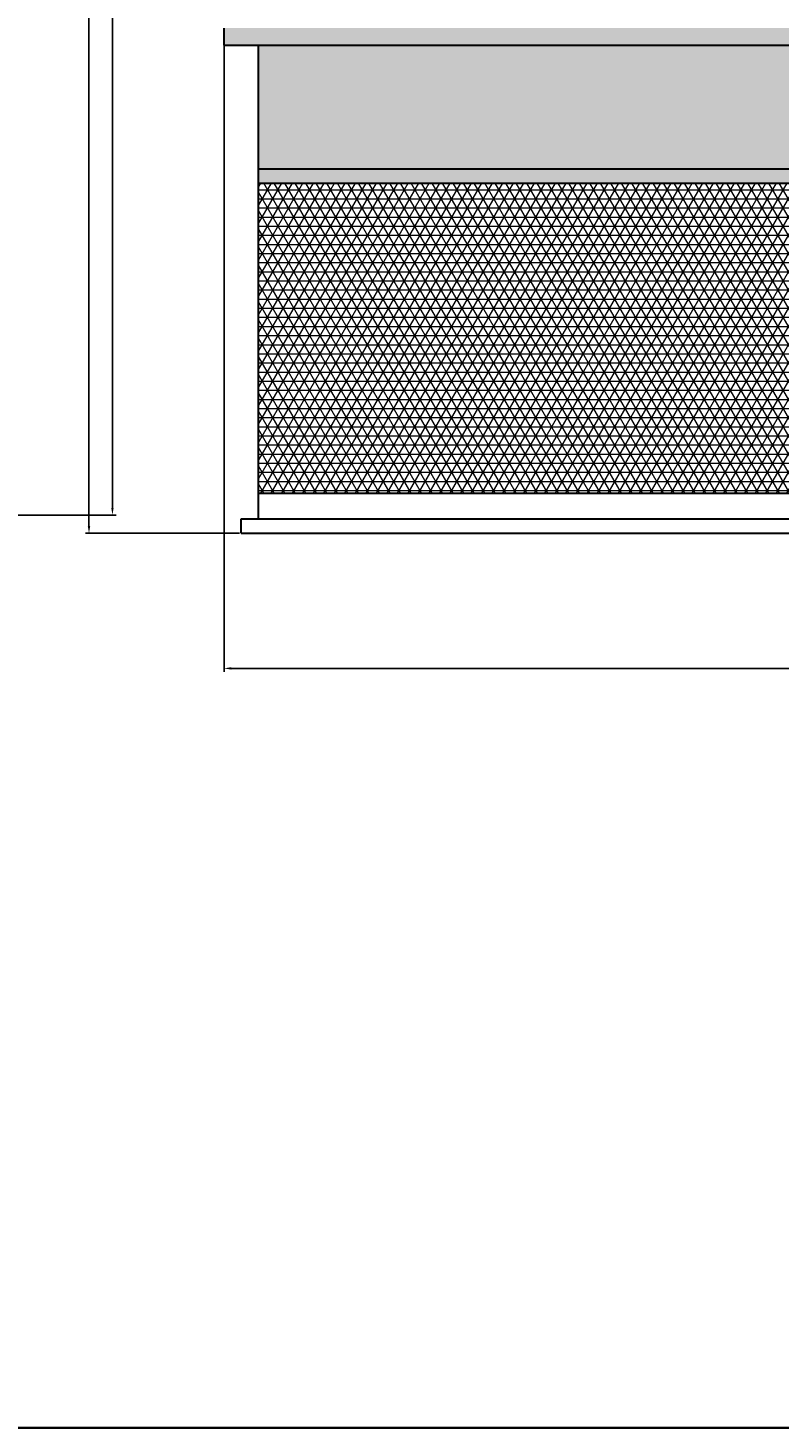
# Model space of a CAD drawing. Units: inches. Extents: x 2391 to 16591, y 7259 to 10239.
# Tile 11 of 27: x 3487 to 3749, y 7259 to 7746. Entities that reach past the tile are written whole.
import ezdxf

# ---------------------------------------------------------------- set-up
doc = ezdxf.new("R2010")
doc.units = ezdxf.units.IN
for name, color, linetype, lineweight in [('A-ANNO-DIMS', 4, 'Continuous', 18), ('A-ANNO-TTLB', 7, 'Continuous', 35), ('A-ELEV', 7, 'Continuous', 30), ('A-ELEV-PATT', 8, 'Continuous', 13), ('A-ELEV-SURF-PATT', 253, 'Continuous', 13)]:
    doc.layers.add(name, color=color, linetype=linetype, lineweight=lineweight)
doc.styles.get("Standard").update_dxf_attribs({"font": 'arial.ttf'})
doc.dimstyles.new('ISO-25', dxfattribs={"dimtxt": 2.5, "dimasz": 2.5, "dimexe": 1.25, "dimexo": 0.625, "dimtad": 1, "dimdec": 0, "dimlunit": 3, "dimtxsty": 'Standard', "dimcen": 2.5, "dimadec": 0, "dimazin": 0, "dimtfac": 1, "dimtdec": 0, "dimtmove": 0, "dimatfit": 3, "dimfxl": 1, "dimarcsym": 0})

# ---------------------------------------------------------------- blocks, each defined once
blk = doc.blocks.new('*D84')
at = {"layer": 'A-ANNO-DIMS', "color": 0, "lineweight": -2, "transparency": 16777216}
for p, q in [((3437.4, 8339.52), (3518.08, 8339.52)), ((3516.83, 7579.02), (3516.83, 8337.02)), ((3464.4, 7576.52), (3518.08, 7576.52))]:
    blk.add_line(p, q, dxfattribs=at)
at = {"layer": 'A-ANNO-DIMS', "color": 0, "transparency": 16777216}
for points in [[(3516.41, 8337.02), (3517.24, 8337.02), (3516.83, 8339.52)], [(3516.41, 7579.02), (3517.24, 7579.02), (3516.83, 7576.52)]]:
    blk.add_solid(points, dxfattribs=at)
at = {"layer": 'Defpoints', "color": 0, "transparency": 16777216}
for p in [(3436.78, 8339.52), (3516.83, 8339.52), (3463.78, 7576.52)]:
    blk.add_point(p, dxfattribs=at)
at = {"layer": 'A-ANNO-DIMS', "color": 0, "transparency": 16777216, "insert": (3514.93, 7958.02), "char_height": 2.5, "attachment_point": 5, "rotation": 90}
blk.add_mtext('63\'-7"', dxfattribs=at)
blk = doc.blocks.new('*D91')
at = {"layer": 'A-ANNO-DIMS', "color": 0, "lineweight": -2, "transparency": 16777216}
for p, q in [((3555.71, 7745.56), (3555.71, 7521.88)), ((4011.71, 7745.56), (4011.71, 7521.88)), ((3558.21, 7523.13), (4009.21, 7523.13))]:
    blk.add_line(p, q, dxfattribs=at)
at = {"layer": 'A-ANNO-DIMS', "color": 0, "transparency": 16777216}
for points in [[(3558.21, 7523.55), (3558.21, 7522.71), (3555.71, 7523.13)], [(4009.21, 7523.55), (4009.21, 7522.71), (4011.71, 7523.13)]]:
    blk.add_solid(points, dxfattribs=at)
at = {"layer": 'Defpoints', "color": 0, "transparency": 16777216}
for p in [(3555.71, 7746.18), (4011.71, 7746.18), (4011.71, 7523.13)]:
    blk.add_point(p, dxfattribs=at)
at = {"layer": 'A-ANNO-DIMS', "color": 0, "transparency": 16777216, "insert": (3783.71, 7525.03), "char_height": 2.5, "attachment_point": 5}
blk.add_mtext('38\'-0"', dxfattribs=at)
blk = doc.blocks.new('*D92')
at = {"layer": 'A-ANNO-DIMS', "color": 0, "lineweight": -2, "transparency": 16777216}
for p, q in [((3777.58, 8333.18), (3507.41, 8333.18)), ((3508.66, 7572.68), (3508.66, 8330.68)), ((3561.08, 7570.18), (3507.41, 7570.18))]:
    blk.add_line(p, q, dxfattribs=at)
at = {"layer": 'A-ANNO-DIMS', "color": 0, "transparency": 16777216}
for points in [[(3508.24, 8330.68), (3509.08, 8330.68), (3508.66, 8333.18)], [(3508.24, 7572.68), (3509.08, 7572.68), (3508.66, 7570.18)]]:
    blk.add_solid(points, dxfattribs=at)
at = {"layer": 'Defpoints', "color": 0, "transparency": 16777216}
for p in [(3508.66, 8333.18), (3778.21, 8333.18), (3561.71, 7570.18)]:
    blk.add_point(p, dxfattribs=at)
at = {"layer": 'A-ANNO-DIMS', "color": 0, "transparency": 16777216, "insert": (3506.76, 7951.68), "char_height": 2.5, "attachment_point": 5, "rotation": 90}
blk.add_mtext('63\'-7"', dxfattribs=at)

msp = doc.modelspace()

# ---------------------------------------------------------------- hatches: boundary and pattern name
at = {"layer": 'A-ELEV-PATT'}
h = msp.add_hatch(dxfattribs=at)
h.set_pattern_fill('BRSTONE', color=256)
h.paths.add_polyline_path([(3999.71, 8226.18), (3881.21, 8226.18), (3881.21, 8070.18), (3999.71, 8070.18)])
h.paths.add_polyline_path([(3956.96, 8118.18), (3914.96, 8118.18), (3914.96, 8172.18), (3956.96, 8172.18)], flags=16)
h.paths.add_polyline_path([(3953.96, 8121.18), (3917.96, 8121.18), (3917.96, 8169.18), (3953.96, 8169.18)], flags=0)
h.paths.add_polyline_path([(3999.71, 8064.18), (3881.21, 8064.18), (3881.21, 7908.18), (3999.71, 7908.18)])
h.paths.add_polyline_path([(3956.96, 7956.18), (3914.96, 7956.18), (3914.96, 8010.18), (3956.96, 8010.18)], flags=16)
h.paths.add_polyline_path([(3953.96, 7959.18), (3917.96, 7959.18), (3917.96, 8007.18), (3953.96, 8007.18)], flags=0)
h.paths.add_polyline_path([(3999.71, 7902.18), (3881.21, 7902.18), (3881.21, 7746.18), (3999.71, 7746.18)])
h.paths.add_polyline_path([(3956.96, 7794.18), (3914.96, 7794.18), (3914.96, 7848.18), (3956.96, 7848.18)], flags=16)
h.paths.add_polyline_path([(3953.96, 7797.18), (3917.96, 7797.18), (3917.96, 7845.18), (3953.96, 7845.18)], flags=0)
h.paths.add_polyline_path([(3999.71, 7740.18), (3567.71, 7740.18), (3567.71, 7697.18), (3760.71, 7697.18), (3760.71, 7706.18), (3755.71, 7706.18), (3755.71, 7711.18), (3774.71, 7711.18), (3774.71, 7706.18), (3769.71, 7706.18), (3769.71, 7677.02), (3772.21, 7677.02), (3772.21, 7679.02), (3774.71, 7679.02), (3774.71, 7704.18), (3843.71, 7704.18), (3843.71, 7589.18), (3774.71, 7589.18), (3774.71, 7584.18), (3913.71, 7584.18), (3913.71, 7589.18), (3844.71, 7589.18), (3844.71, 7704.18), (3913.71, 7704.18), (3913.71, 7679.02), (3916.21, 7679.02), (3916.21, 7677.02), (3918.71, 7677.02), (3918.71, 7706.18), (3913.71, 7706.18), (3913.71, 7711.18), (3932.71, 7711.18), (3932.71, 7706.18), (3927.71, 7706.18), (3927.71, 7697.18), (3999.71, 7697.18)])
h.paths.add_polyline_path([(3918.71, 7675.02), (3916.21, 7675.02), (3916.21, 7673.02), (3913.71, 7673.02), (3913.71, 7618.89), (3916.21, 7618.89), (3916.21, 7616.89), (3918.71, 7616.89)], flags=17)
h.paths.add_polyline_path([(3918.71, 7614.89), (3916.21, 7614.89), (3916.21, 7612.89), (3913.71, 7612.89), (3913.71, 7584.18), (3918.71, 7584.18)], flags=17)
h.paths.add_polyline_path([(3774.71, 7673.02), (3772.21, 7673.02), (3772.21, 7675.02), (3769.71, 7675.02), (3769.71, 7616.89), (3772.21, 7616.89), (3772.21, 7618.89), (3774.71, 7618.89)], flags=17)
h.paths.add_polyline_path([(3774.71, 7612.89), (3772.21, 7612.89), (3772.21, 7614.89), (3769.71, 7614.89), (3769.71, 7584.18), (3774.71, 7584.18), (3774.71, 7589.18)], flags=17)
h = msp.add_hatch(dxfattribs=at)
h.set_pattern_fill('NET3', color=256)
h.paths.add_polyline_path([(3760.71, 7692.18), (3567.71, 7692.18), (3567.71, 7584.18), (3760.71, 7584.18)])
h.paths.add_polyline_path([(3999.71, 7692.18), (3927.71, 7692.18), (3927.71, 7584.18), (3999.71, 7584.18)])
at = {"layer": 'A-ELEV-SURF-PATT'}
h = msp.add_hatch(color=256, dxfattribs=at)
h.dxf.hatch_style = 1
h.paths.add_polyline_path([(4011.71, 7740.18), (4011.71, 7746.18), (3555.71, 7746.18), (3555.71, 7740.18)])
h.paths.add_polyline_path([(4011.71, 7902.18), (4011.71, 7908.18), (3555.71, 7908.18), (3555.71, 7902.18)])
h.paths.add_polyline_path([(4011.71, 8064.18), (4011.71, 8070.18), (3555.71, 8070.18), (3555.71, 8064.18)])
h.paths.add_polyline_path([(3555.71, 8232.18), (3555.71, 8226.18), (4011.71, 8226.18), (4011.71, 8232.18)])
h.paths.add_polyline_path([(3778.21, 8333.18), (3778.21, 8328.18), (3978.71, 8328.18), (3978.71, 8333.18)])
h = msp.add_hatch(color=256, dxfattribs=at)
h.dxf.hatch_style = 1
h.paths.add_polyline_path([(3760.71, 7692.18), (3760.71, 7697.18), (3567.71, 7697.18), (3567.71, 7692.18)])
h.paths.add_polyline_path([(3755.71, 7711.18), (3755.71, 7706.18), (3774.71, 7706.18), (3774.71, 7711.18)])
h.paths.add_polyline_path([(3913.71, 7711.18), (3913.71, 7706.18), (3932.71, 7706.18), (3932.71, 7711.18)])
h.paths.add_polyline_path([(3927.71, 7697.18), (3927.71, 7692.18), (3999.71, 7692.18), (3999.71, 7697.18)])

# ---------------------------------------------------------------- linework, layer by layer
at = {"layer": 'A-ANNO-TTLB'}
msp.add_lwpolyline([(2391.28, 10239.38), (4154.2, 10239.38), (4154.2, 7258.54), (2391.28, 7258.54)], close=True, dxfattribs=at)
at = {"layer": 'A-ELEV'}
for p, q in [((3555.71, 7740.18), (3555.71, 7746.18)), ((3555.71, 7740.18), (4011.71, 7740.18)), ((3567.71, 7575.18), (3567.71, 7740.18)), ((3567.71, 7697.18), (3760.71, 7697.18)), ((3567.71, 7692.18), (3760.71, 7692.18)), ((3567.71, 7584.18), (3999.71, 7584.18)), ((3561.71, 7570.18), (3561.71, 7575.18)), ((3561.71, 7575.18), (4005.71, 7575.18)), ((3561.71, 7570.18), (4005.71, 7570.18))]:
    msp.add_line(p, q, dxfattribs=at)

# ---------------------------------------------------------------- dimensions: what is measured, and where the dimension line sits
at = {"layer": 'A-ANNO-DIMS'}
for base, p1, p2, picture, middle in [((3516.83, 8339.52), (3463.78, 7576.52), (3436.78, 8339.52), '*D84', (3514.93, 7958.02)), ((3508.66, 8333.18), (3561.71, 7570.18), (3778.21, 8333.18), '*D92', (3506.76, 7951.68))]:
    dim = msp.add_linear_dim(base=base, p1=p1, p2=p2, angle=90, dimstyle='ISO-25', override={"dimdec": 1, "dimlfac": 1, "dimrnd": 0, "dimzin": 1, "dimdsep": 46, "dimlunit": 4, "dimfrac": 2}, dxfattribs=at)
    dim.commit()
    dim.dimension.update_dxf_attribs({"geometry": picture, "text_midpoint": middle})
dim = msp.add_linear_dim(base=(4011.71, 7523.13), p1=(3555.71, 7746.18), p2=(4011.71, 7746.18), dimstyle='ISO-25', override={"dimdec": 1, "dimlfac": 1, "dimrnd": 0, "dimzin": 1, "dimdsep": 46, "dimlunit": 4, "dimfrac": 2}, dxfattribs=at)
dim.commit()
dim.dimension.update_dxf_attribs({"geometry": '*D91', "text_midpoint": (3783.71, 7525.03)})

doc.saveas('drawing.dxf')
